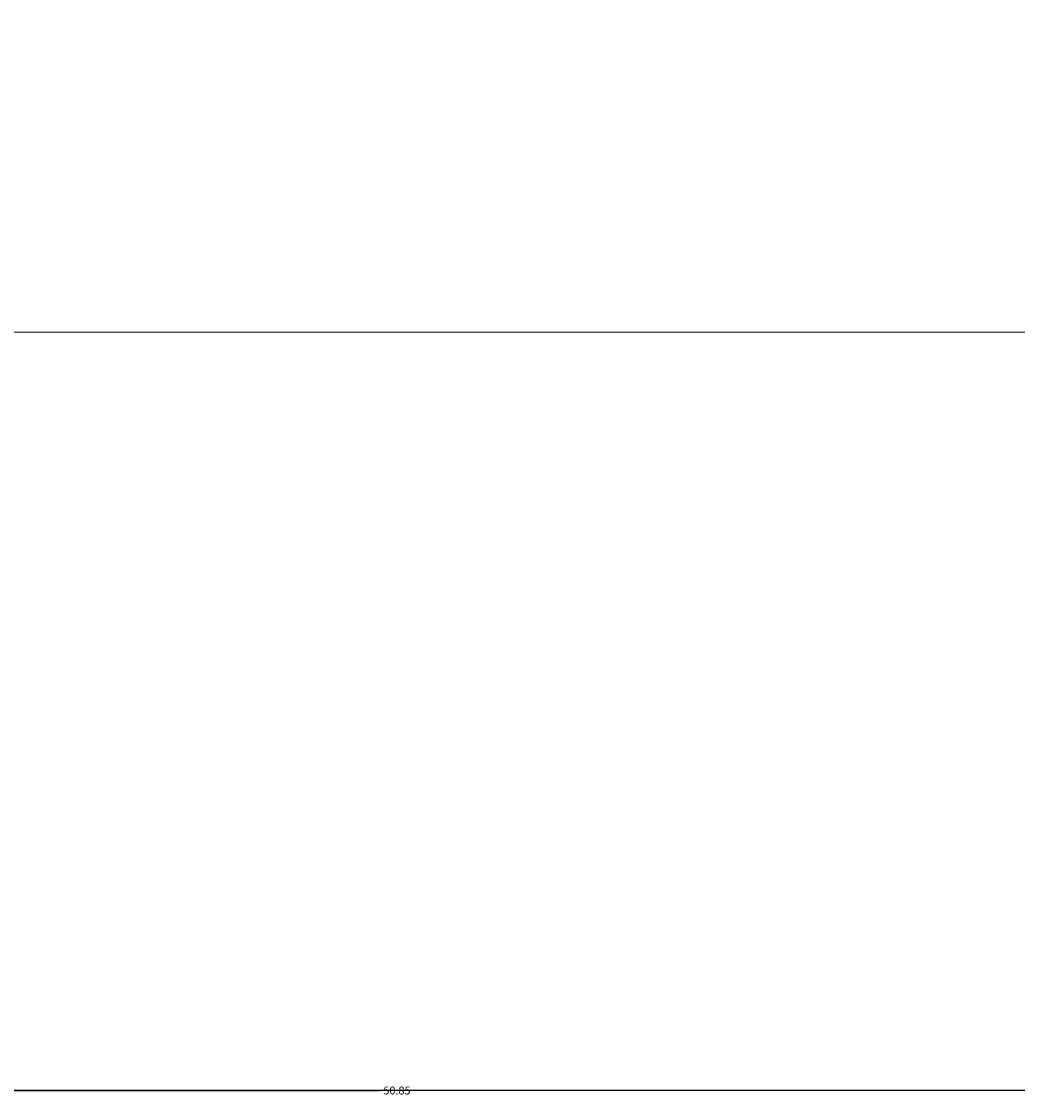
# Model space of a CAD drawing. Units: inches. Extents: x 412 to 584, y 208 to 437.
# Tile 7 of 28: x 516 to 539, y 208 to 233. Entities that reach past the tile are written whole.
import ezdxf

# ---------------------------------------------------------------- set-up
doc = ezdxf.new("R2010")
doc.units = ezdxf.units.IN
doc.header["$MEASUREMENT"] = 0
doc.layers.add('A-ANNO-DIMS', color=2, linetype='Continuous', lineweight=18)
doc.layers.add('E-ENCL', color=8, linetype='Continuous', lineweight=18)
doc.styles.get("Standard").update_dxf_attribs({"font": 'arial.ttf'})
doc.dimstyles.get("Standard").update_dxf_attribs({"dimtxt": 0.18, "dimasz": 0.18, "dimexe": 0.18, "dimexo": 0.0625, "dimgap": 0.09, "dimtad": 0, "dimtih": 1, "dimtoh": 1, "dimdec": 4, "dimzin": 0, "dimdsep": 46, "dimtxsty": 'Standard', "dimcen": 0.09, "dimadec": 0, "dimazin": 0, "dimtfac": 1, "dimtdec": 4, "dimtofl": 0, "dimtmove": 0, "dimatfit": 3, "dimfxl": 1, "dimtolj": 1, "dimtzin": 0, "dimarcsym": 0})

# ---------------------------------------------------------------- blocks, each defined once
blk = doc.blocks.new('*D13')
at = {"layer": 'A-ANNO-DIMS', "color": 0, "lineweight": -2, "transparency": 16777216}
for p, q in [((423.556, 225.526), (423.556, 208.233)), ((572.394, 225.526), (572.394, 208.233)), ((423.736, 208.413), (497.52, 208.413)), ((572.214, 208.413), (498.43, 208.413))]:
    blk.add_line(p, q, dxfattribs=at)
at = {"layer": 'A-ANNO-DIMS', "color": 0, "transparency": 16777216}
for points in [[(423.736, 208.443), (423.736, 208.383), (423.556, 208.413)], [(572.214, 208.443), (572.214, 208.383), (572.394, 208.413)]]:
    blk.add_solid(points, dxfattribs=at)
at = {"layer": 'Defpoints', "color": 0, "transparency": 16777216}
for p in [(423.556, 225.588), (572.394, 225.588), (572.394, 208.413)]:
    blk.add_point(p, dxfattribs=at)
at = {"layer": 'A-ANNO-DIMS', "color": 0, "transparency": 16777216, "insert": (497.975, 208.413), "char_height": 0.18, "attachment_point": 5}
blk.add_mtext('\\A1;148.84', dxfattribs=at)
blk = doc.blocks.new('*D16')
at = {"layer": 'A-ANNO-DIMS', "color": 0, "lineweight": -2, "transparency": 16777216}
for p, q in [((499.288, 219.47), (499.288, 208.233)), ((550.135, 219.451), (550.135, 208.233)), ((499.468, 208.413), (524.317, 208.413)), ((549.955, 208.413), (525.106, 208.413))]:
    blk.add_line(p, q, dxfattribs=at)
at = {"layer": 'A-ANNO-DIMS', "color": 0, "transparency": 16777216}
for points in [[(499.468, 208.443), (499.468, 208.383), (499.288, 208.413)], [(549.955, 208.443), (549.955, 208.383), (550.135, 208.413)]]:
    blk.add_solid(points, dxfattribs=at)
at = {"layer": 'Defpoints', "color": 0, "transparency": 16777216}
for p in [(499.288, 219.533), (550.135, 219.513), (550.135, 208.413)]:
    blk.add_point(p, dxfattribs=at)
at = {"layer": 'A-ANNO-DIMS', "color": 0, "transparency": 16777216, "insert": (524.711, 208.413), "char_height": 0.18, "attachment_point": 5}
blk.add_mtext('\\A1;50.85', dxfattribs=at)
blk = doc.blocks.new('*D17')
at = {"layer": 'A-ANNO-DIMS', "color": 0, "lineweight": -2, "transparency": 16777216}
for p, q in [((497.715, 426.185), (583.674, 426.185)), ((583.494, 426.005), (583.494, 323.031)), ((583.494, 219.693), (583.494, 322.667)), ((550.198, 219.513), (583.674, 219.513))]:
    blk.add_line(p, q, dxfattribs=at)
at = {"layer": 'A-ANNO-DIMS', "color": 0, "transparency": 16777216}
for points in [[(583.464, 426.005), (583.524, 426.005), (583.494, 426.185)], [(583.464, 219.693), (583.524, 219.693), (583.494, 219.513)]]:
    blk.add_solid(points, dxfattribs=at)
at = {"layer": 'Defpoints', "color": 0, "transparency": 16777216}
for p in [(497.652, 426.185), (550.135, 219.513), (583.494, 219.513)]:
    blk.add_point(p, dxfattribs=at)
at = {"layer": 'A-ANNO-DIMS', "color": 0, "transparency": 16777216, "insert": (583.494, 322.849), "char_height": 0.18, "attachment_point": 5}
blk.add_mtext('\\A1;206.67', dxfattribs=at)

msp = doc.modelspace()

# ---------------------------------------------------------------- linework, layer by layer
at = {"layer": 'E-ENCL'}
msp.add_lwpolyline([(423.5562, 309.3773), (572.3937, 309.3773), (572.3937, 225.5881), (423.5562, 225.5881)], close=True, dxfattribs=at)

# ---------------------------------------------------------------- dimensions: what is measured, and where the dimension line sits
at = {"layer": 'A-ANNO-DIMS'}
dim = msp.add_linear_dim(base=(583.4937, 219.5133), p1=(497.6523, 426.1847), p2=(550.1351, 219.5133), angle=90, dimstyle='Standard', override={"dimdec": 2, "dimlfac": 1, "dimrnd": 0, "dimzin": 0, "dimdsep": 46, "dimlunit": 2}, dxfattribs=at)
dim.commit()
dim.dimension.update_dxf_attribs({"geometry": '*D17', "text_midpoint": (583.4937, 322.849)})
for base, p1, p2, picture, middle in [((572.3937, 208.4133), (423.5562, 225.5881), (572.3937, 225.5881), '*D13', (497.975, 208.4133)), ((550.1351, 208.4133), (499.2878, 219.5329), (550.1351, 219.5133), '*D16', (524.7115, 208.4133))]:
    dim = msp.add_linear_dim(base=base, p1=p1, p2=p2, dimstyle='Standard', override={"dimdec": 2, "dimlfac": 1, "dimrnd": 0, "dimzin": 0, "dimdsep": 46, "dimlunit": 2}, dxfattribs=at)
    dim.commit()
    dim.dimension.update_dxf_attribs({"geometry": picture, "text_midpoint": middle})

doc.saveas('drawing.dxf')
